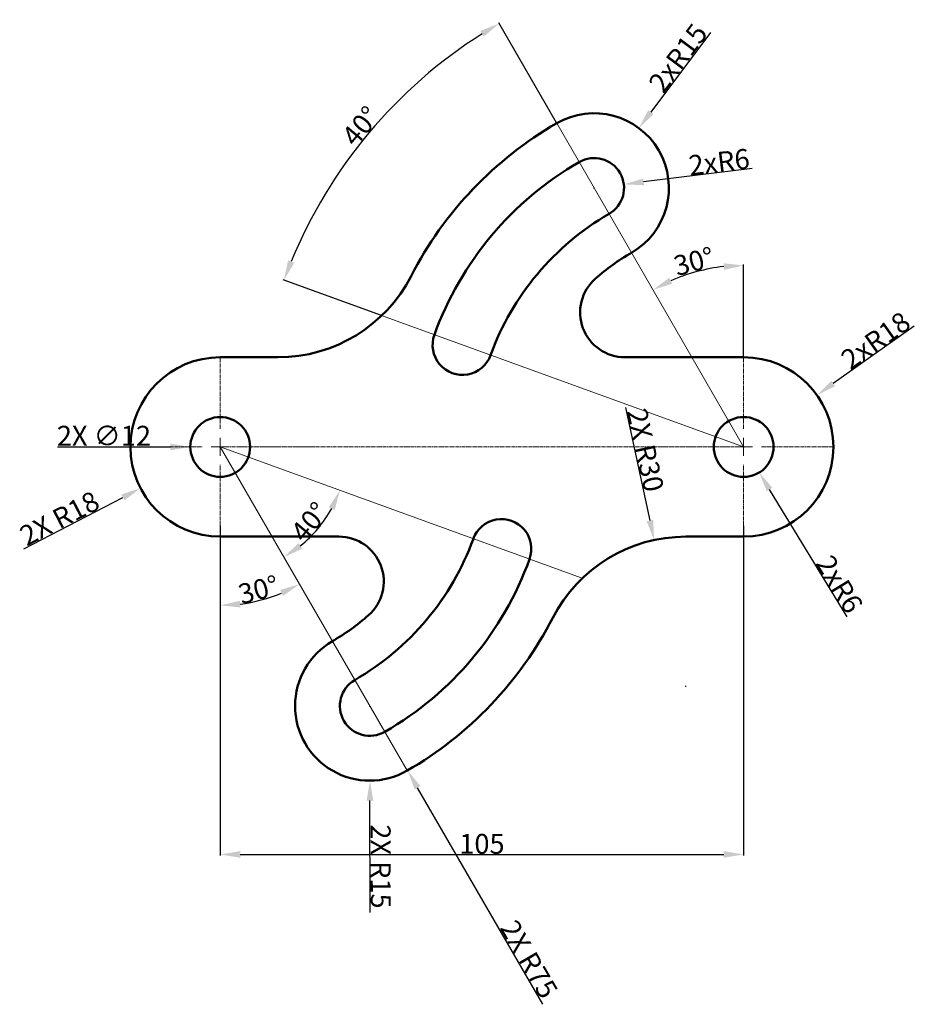
# Model space of a CAD drawing. Units: millimetres. Extents: x 75 to 254, y -22 to 175.
import ezdxf

# ---------------------------------------------------------------- set-up
doc = ezdxf.new("R2010")
doc.units = ezdxf.units.MM
doc.header["$MEASUREMENT"] = 0
doc.linetypes.add('CENTER2', pattern=[1.125, 0.75, -0.125, 0.125, -0.125])
for name, color, linetype, lineweight in [('M-CNTR', 8, 'CENTER2', 18), ('M-CONS', 8, 'Continuous', 13), ('M-DIMS', 2, 'Continuous', 25), ('M-OUTL', 7, 'Continuous', 50)]:
    doc.layers.add(name, color=color, linetype=linetype, lineweight=lineweight)
doc.styles.get("Standard").update_dxf_attribs({"font": 'arial.ttf'})
doc.dimstyles.get("Standard").update_dxf_attribs({"dimtxt": 4, "dimasz": 4, "dimexe": 0.18, "dimexo": 0.0625, "dimgap": 0.09, "dimtad": 1, "dimdec": 0, "dimzin": 0, "dimdsep": 46, "dimtxsty": 'Standard', "dimcen": 0.09, "dimclre": 251, "dimadec": 0, "dimazin": 0, "dimtfac": 1, "dimtdec": 0, "dimtofl": 0, "dimtmove": 0, "dimatfit": 3, "dimfxl": 1, "dimtolj": 1, "dimtzin": 0, "dimarcsym": 0})

# ---------------------------------------------------------------- blocks, each defined once
blk = doc.blocks.new('*U1')
at = {"layer": 'M-CNTR', "color": 0, "transparency": 16777216}
for p, q in [((0, 3.6), (0, 18.12)), ((-18.12, 0), (-3.6, 0)), ((3.6, 0), (18.12, 0)), ((0, -18.12), (0, -3.6))]:
    blk.add_line(p, q, dxfattribs=at)
at = {"layer": 'M-CNTR', "color": 0, "linetype": 'Continuous', "transparency": 16777216}
for p, q in [((-1.8, 0), (1.8, 0)), ((0, -1.8), (0, 1.8))]:
    blk.add_line(p, q, dxfattribs=at)
blk = doc.blocks.new('*U2')
at = {"layer": 'M-CNTR', "color": 0, "transparency": 16777216}
for p, q in [((0, 3.6), (0, 18.12)), ((-18.12, 0), (-3.6, 0)), ((3.6, 0), (18.12, 0)), ((0, -18.12), (0, -3.6))]:
    blk.add_line(p, q, dxfattribs=at)
at = {"layer": 'M-CNTR', "color": 0, "linetype": 'Continuous', "transparency": 16777216}
for p, q in [((-1.8, 0), (1.8, 0)), ((0, -1.8), (0, 1.8))]:
    blk.add_line(p, q, dxfattribs=at)
blk = doc.blocks.new('*D3')
at = {"layer": 'Defpoints', "color": 0, "transparency": 16777216}
for p in [(152.62, 160.91), (182.47, 154.53), (147.35, 115.92), (219.97, 89.58), (219.97, 89.58)]:
    blk.add_point(p, dxfattribs=at)
at = {"layer": 'M-DIMS', "color": 0, "lineweight": -2, "transparency": 16777216}
for p, q in [((182.44, 154.58), (170.83, 174.69)), ((147.29, 115.94), (127.58, 123.09))]:
    blk.add_line(p, q, dxfattribs=at)
blk.add_arc((219.97, 89.58), 98.1, 122.3363, 157.7248, dxfattribs=at)
at = {"layer": 'M-DIMS', "color": 0, "transparency": 16777216}
for points in [[(167.15, 173.04), (167.84, 171.9), (170.92, 174.54)], [(129.81, 126.52), (128.57, 127), (127.75, 123.03)]]:
    blk.add_solid(points, dxfattribs=at)
at = {"layer": 'M-DIMS', "color": 0, "transparency": 16777216, "insert": (143.15, 153.97), "char_height": 4, "attachment_point": 5, "rotation": 50.0305}
blk.add_mtext('\\A1;40°', dxfattribs=at)
blk = doc.blocks.new('*D4')
at = {"layer": 'Defpoints', "color": 0, "transparency": 16777216}
for p in [(114.97, 89.58), (114.97, 85.98), (114.97, 71.46), (120.49, 58.27), (152.47, 24.63)]:
    blk.add_point(p, dxfattribs=at)
at = {"layer": 'M-DIMS', "color": 0, "lineweight": -2, "transparency": 16777216}
blk.add_line((114.97, 71.39), (114.97, 57.61), dxfattribs=at)
blk.add_arc((114.97, 89.58), 31.79, 277.2151, 292.7849, dxfattribs=at)
at = {"layer": 'M-DIMS', "color": 0, "transparency": 16777216}
for points in [[(126.99, 60.87), (127.58, 59.68), (130.86, 62.05)], [(119.01, 57.38), (118.92, 58.71), (114.97, 57.79)]]:
    blk.add_solid(points, dxfattribs=at)
at = {"layer": 'M-DIMS', "color": 0, "transparency": 16777216, "insert": (122.65, 60.94), "char_height": 4, "attachment_point": 5, "rotation": 15}
blk.add_mtext('\\A1;30°', dxfattribs=at)
blk = doc.blocks.new('*D5')
at = {"layer": 'Defpoints', "color": 0, "transparency": 16777216}
for p in [(114.97, 89.58), (114.97, 89.58), (132.5, 71.01), (187.6, 63.23), (152.47, 24.63)]:
    blk.add_point(p, dxfattribs=at)
at = {"layer": 'M-DIMS', "color": 0, "lineweight": -2, "transparency": 16777216}
blk.add_arc((114.97, 89.58), 25.54, 308.9834, 331.0777, dxfattribs=at)
at = {"layer": 'M-DIMS', "color": 0, "transparency": 16777216}
for points in [[(136.72, 77.5), (137.93, 76.95), (138.98, 80.87)], [(131.42, 69.18), (130.66, 70.28), (127.74, 67.46)]]:
    blk.add_solid(points, dxfattribs=at)
at = {"layer": 'M-DIMS', "color": 0, "transparency": 16777216, "insert": (132.91, 74.54), "char_height": 4, "attachment_point": 5, "rotation": 50.0305}
blk.add_mtext('\\A1;40°', dxfattribs=at)
blk = doc.blocks.new('*D6')
at = {"layer": 'Defpoints', "color": 0, "transparency": 16777216}
for p in [(114.97, 73.82), (219.97, 73.82), (219.97, 7.81)]:
    blk.add_point(p, dxfattribs=at)
at = {"layer": 'M-DIMS', "color": 0, "lineweight": -2, "transparency": 16777216}
for p, q in [((114.97, 73.75), (114.97, 7.63)), ((219.97, 73.75), (219.97, 7.63)), ((118.97, 7.81), (215.97, 7.81))]:
    blk.add_line(p, q, dxfattribs=at)
at = {"layer": 'M-DIMS', "color": 0, "transparency": 16777216}
for points in [[(118.97, 8.48), (118.97, 7.15), (114.97, 7.81)], [(215.97, 8.48), (215.97, 7.15), (219.97, 7.81)]]:
    blk.add_solid(points, dxfattribs=at)
at = {"layer": 'M-DIMS', "color": 0, "transparency": 16777216, "insert": (167.47, 9.94), "char_height": 4, "attachment_point": 5}
blk.add_mtext('\\A1;105', dxfattribs=at)
blk = doc.blocks.new('*D7')
at = {"layer": 'Defpoints', "color": 0, "transparency": 16777216}
for p in [(234.66, 99.98), (219.97, 89.58)]:
    blk.add_point(p, dxfattribs=at)
at = {"layer": 'M-DIMS', "color": 0, "lineweight": -2, "transparency": 16777216}
for p, q in [((254.18, 113.81), (237.93, 102.29)), ((219.88, 89.58), (220.06, 89.58)), ((219.97, 89.49), (219.97, 89.67))]:
    blk.add_line(p, q, dxfattribs=at)
at = {"layer": 'M-DIMS', "color": 0, "transparency": 16777216}
blk.add_solid([(237.54, 102.84), (238.31, 101.75), (234.66, 99.98)], dxfattribs=at)
at = {"layer": 'M-DIMS', "color": 0, "transparency": 16777216, "insert": (246.45, 110.95), "char_height": 4, "attachment_point": 5, "rotation": 35.3084}
blk.add_mtext('\\A1;2xR18', dxfattribs=at)
blk = doc.blocks.new('*D8')
at = {"layer": 'Defpoints', "color": 0, "transparency": 16777216}
for p in [(219.97, 89.58), (223.09, 84.45)]:
    blk.add_point(p, dxfattribs=at)
at = {"layer": 'M-DIMS', "color": 0, "lineweight": -2, "transparency": 16777216}
for p, q in [((219.88, 89.58), (220.06, 89.58)), ((219.97, 89.49), (219.97, 89.67)), ((240.72, 55.46), (225.17, 81.03))]:
    blk.add_line(p, q, dxfattribs=at)
at = {"layer": 'M-DIMS', "color": 0, "transparency": 16777216}
blk.add_solid([(225.74, 81.38), (224.6, 80.69), (223.09, 84.45)], dxfattribs=at)
at = {"layer": 'M-DIMS', "color": 0, "transparency": 16777216, "insert": (239.21, 62.04), "char_height": 4, "attachment_point": 5, "rotation": 301.3002}
blk.add_mtext('\\A1;2xR6', dxfattribs=at)
blk = doc.blocks.new('*D9')
at = {"layer": 'Defpoints', "color": 0, "transparency": 16777216}
for p in [(182.47, 154.53), (213.65, 125.43), (219.97, 107.7), (219.97, 93.18), (219.97, 89.58)]:
    blk.add_point(p, dxfattribs=at)
at = {"layer": 'M-DIMS', "color": 0, "lineweight": -2, "transparency": 16777216}
blk.add_line((219.97, 107.76), (219.97, 126.17), dxfattribs=at)
blk.add_arc((219.97, 89.58), 36.41, 96.2977, 113.7023, dxfattribs=at)
at = {"layer": 'M-DIMS', "color": 0, "transparency": 16777216}
for points in [[(215.94, 126.43), (216.01, 125.1), (219.97, 125.99)], [(205.64, 122.32), (205.03, 123.51), (201.77, 121.11)]]:
    blk.add_solid(points, dxfattribs=at)
at = {"layer": 'M-DIMS', "color": 0, "transparency": 16777216, "insert": (210, 126.81), "char_height": 4, "attachment_point": 5, "rotation": 15}
blk.add_mtext('\\A1;30°', dxfattribs=at)
blk = doc.blocks.new('*D10')
at = {"layer": 'Defpoints', "color": 0, "transparency": 16777216}
for p in [(198.96, 153.55), (189.97, 141.54)]:
    blk.add_point(p, dxfattribs=at)
at = {"layer": 'M-DIMS', "color": 0, "lineweight": -2, "transparency": 16777216}
for p, q in [((213.3, 172.73), (201.35, 156.75)), ((189.88, 141.54), (190.06, 141.54)), ((189.97, 141.45), (189.97, 141.63))]:
    blk.add_line(p, q, dxfattribs=at)
at = {"layer": 'M-DIMS', "color": 0, "transparency": 16777216}
blk.add_solid([(200.82, 157.15), (201.88, 156.36), (198.96, 153.55)], dxfattribs=at)
at = {"layer": 'M-DIMS', "color": 0, "transparency": 16777216, "insert": (206.81, 167.62), "char_height": 4, "attachment_point": 5, "rotation": 53.2096}
blk.add_mtext('\\A1;2xR15', dxfattribs=at)
blk = doc.blocks.new('*D11')
at = {"layer": 'Defpoints', "color": 0, "transparency": 16777216}
for p in [(195.93, 142.27), (189.97, 141.54)]:
    blk.add_point(p, dxfattribs=at)
at = {"layer": 'M-DIMS', "color": 0, "lineweight": -2, "transparency": 16777216}
for p, q in [((221.66, 145.42), (199.9, 142.76)), ((189.88, 141.54), (190.06, 141.54)), ((189.97, 141.45), (189.97, 141.63))]:
    blk.add_line(p, q, dxfattribs=at)
at = {"layer": 'M-DIMS', "color": 0, "transparency": 16777216}
blk.add_solid([(199.82, 143.42), (199.98, 142.09), (195.93, 142.27)], dxfattribs=at)
at = {"layer": 'M-DIMS', "color": 0, "transparency": 16777216, "insert": (215.05, 146.76), "char_height": 4, "attachment_point": 5, "rotation": 6.9895}
blk.add_mtext('\\A1;2xR6', dxfattribs=at)
blk = doc.blocks.new('SLOT-ARC-R60-W12')
for centre, radius, start, end in [((32.4, 37.5), 6, 300, 120), ((62.4, -14.46), 66, 120, 160.0611), ((62.4, -14.46), 54, 120, 160.0611), ((6, 6), 6, 160.0611, 340.0611)]:
    blk.add_arc(centre, radius, start, end)
blk = doc.blocks.new('*D13')
at = {"layer": 'Defpoints', "color": 0, "transparency": 16777216}
for p in [(114.97, 89.58), (152.55, 24.67)]:
    blk.add_point(p, dxfattribs=at)
at = {"layer": 'M-DIMS', "color": 251, "lineweight": -2, "transparency": 16777216}
for p, q in [((114.88, 89.58), (115.06, 89.58)), ((114.97, 89.49), (114.97, 89.67))]:
    blk.add_line(p, q, dxfattribs=at)
at = {"layer": 'M-DIMS', "color": 0, "lineweight": -2, "transparency": 16777216}
blk.add_line((179.71, -22.25), (154.55, 21.21), dxfattribs=at)
at = {"layer": 'M-DIMS', "color": 0, "transparency": 16777216}
blk.add_solid([(155.13, 21.54), (153.97, 20.87), (152.55, 24.67)], dxfattribs=at)
at = {"layer": 'M-DIMS', "color": 0, "transparency": 16777216, "insert": (176.93, -13.21), "char_height": 4, "attachment_point": 5, "rotation": 300.0647}
blk.add_mtext('\\A1;2X R75', dxfattribs=at)
blk = doc.blocks.new('*D14')
at = {"layer": 'Defpoints', "color": 0, "transparency": 16777216}
for p in [(202.01, 70.9), (208.36, 41.58)]:
    blk.add_point(p, dxfattribs=at)
at = {"layer": 'M-DIMS', "color": 0, "lineweight": -2, "transparency": 16777216}
blk.add_line((196.26, 97.48), (201.16, 74.81), dxfattribs=at)
at = {"layer": 'M-DIMS', "color": 251, "lineweight": -2, "transparency": 16777216}
for p, q in [((208.27, 41.58), (208.45, 41.58)), ((208.36, 41.49), (208.36, 41.67))]:
    blk.add_line(p, q, dxfattribs=at)
at = {"layer": 'M-DIMS', "color": 0, "transparency": 16777216}
blk.add_solid([(201.82, 74.95), (200.51, 74.67), (202.01, 70.9)], dxfattribs=at)
at = {"layer": 'M-DIMS', "color": 0, "transparency": 16777216, "insert": (200.29, 88.94), "char_height": 4, "attachment_point": 5, "rotation": 282.2146}
blk.add_mtext('\\A1;2X R30', dxfattribs=at)
blk = doc.blocks.new('*D15')
at = {"layer": 'Defpoints', "color": 0, "transparency": 16777216}
for p in [(108.97, 89.58), (120.97, 89.58)]:
    blk.add_point(p, dxfattribs=at)
at = {"layer": 'M-DIMS', "color": 0, "lineweight": -2, "transparency": 16777216}
blk.add_line((82.3, 89.58), (104.97, 89.58), dxfattribs=at)
at = {"layer": 'M-DIMS', "color": 251, "lineweight": -2, "transparency": 16777216}
for p, q in [((114.88, 89.58), (115.06, 89.58)), ((114.97, 89.49), (114.97, 89.67))]:
    blk.add_line(p, q, dxfattribs=at)
at = {"layer": 'M-DIMS', "color": 0, "transparency": 16777216}
blk.add_solid([(104.97, 90.24), (104.97, 88.91), (108.97, 89.58)], dxfattribs=at)
at = {"layer": 'M-DIMS', "color": 0, "transparency": 16777216, "insert": (91.64, 91.82), "char_height": 4, "attachment_point": 5, "rotation": 0.003}
blk.add_mtext('\\A1;2X ∅12', dxfattribs=at)
blk = doc.blocks.new('*D16')
at = {"layer": 'Defpoints', "color": 0, "transparency": 16777216}
for p in [(114.97, 89.58), (98.99, 81.3)]:
    blk.add_point(p, dxfattribs=at)
at = {"layer": 'M-DIMS', "color": 251, "lineweight": -2, "transparency": 16777216}
for p, q in [((114.88, 89.58), (115.06, 89.58)), ((114.97, 89.49), (114.97, 89.67))]:
    blk.add_line(p, q, dxfattribs=at)
at = {"layer": 'M-DIMS', "color": 0, "lineweight": -2, "transparency": 16777216}
blk.add_line((75.54, 69.14), (95.44, 79.45), dxfattribs=at)
at = {"layer": 'M-DIMS', "color": 0, "transparency": 16777216}
blk.add_solid([(95.13, 80.05), (95.75, 78.86), (98.99, 81.3)], dxfattribs=at)
at = {"layer": 'M-DIMS', "color": 0, "transparency": 16777216, "insert": (82.73, 75.27), "char_height": 4, "attachment_point": 5, "rotation": 27.3947}
blk.add_mtext('\\A1;2X R18', dxfattribs=at)
blk = doc.blocks.new('*D17')
at = {"layer": 'Defpoints', "color": 0, "transparency": 16777216}
for p in [(144.97, 37.62), (145, 22.62)]:
    blk.add_point(p, dxfattribs=at)
at = {"layer": 'M-DIMS', "color": 251, "lineweight": -2, "transparency": 16777216}
for p, q in [((144.88, 37.62), (145.06, 37.62)), ((144.97, 37.53), (144.97, 37.71))]:
    blk.add_line(p, q, dxfattribs=at)
at = {"layer": 'M-DIMS', "color": 0, "lineweight": -2, "transparency": 16777216}
blk.add_line((145.05, -3.82), (145.01, 18.62), dxfattribs=at)
at = {"layer": 'M-DIMS', "color": 0, "transparency": 16777216}
blk.add_solid([(145.67, 18.62), (144.34, 18.61), (145, 22.62)], dxfattribs=at)
at = {"layer": 'M-DIMS', "color": 0, "transparency": 16777216, "insert": (147.16, 5.4), "char_height": 4, "attachment_point": 5, "rotation": 270.1063}
blk.add_mtext('\\A1;2X R15', dxfattribs=at)

msp = doc.modelspace()

# ---------------------------------------------------------------- linework, layer by layer
at = {"layer": 'M-CNTR'}
msp.add_line((114.97, 89.58), (219.97, 89.58), dxfattribs=at)
at = {"layer": 'M-CONS'}
for p, q in [((219.97, 89.58), (182.47, 154.53)), ((219.97, 89.58), (147.35, 115.92)), ((114.97, 89.58), (152.47, 24.63)), ((114.97, 89.58), (187.6, 63.23))]:
    msp.add_line(p, q, dxfattribs=at)
at = {"layer": 'M-OUTL'}
for p, q in [((114.97, 107.58), (126.59, 107.58)), ((219.97, 107.58), (196.16, 107.58)), ((114.97, 71.58), (138.78, 71.58)), ((219.97, 71.58), (208.36, 71.58))]:
    msp.add_line(p, q, dxfattribs=at)
for centre in [(114.97, 89.58), (219.97, 89.58)]:
    msp.add_circle(centre, 6, dxfattribs=at)
for centre, radius, start, end in [((189.97, 141.54), 15, 300, 120), ((219.97, 89.58), 75, 120, 152.7971), ((219.97, 89.58), 45, 120, 131.4096), ((126.59, 137.58), 30, 270, 332.7971), ((196.16, 116.58), 9, 131.4096, 270), ((114.97, 89.58), 18, 90, 270), ((219.97, 89.58), 18, 270, 90), ((138.78, 62.58), 9, 311.4096, 90), ((208.36, 41.58), 30, 90, 152.7971), ((114.97, 89.58), 45, 300, 311.4096), ((114.97, 89.58), 75, 300, 332.7971), ((144.97, 37.62), 15, 120, 300)]:
    msp.add_arc(centre, radius, start, end, dxfattribs=at)

# ---------------------------------------------------------------- block references
at = {"layer": 'M-CNTR'}
for name, p in [('*U1', (114.97, 89.58)), ('*U2', (219.97, 89.58))]:
    msp.add_blockref(name, p, dxfattribs=at)
at = {"layer": 'M-OUTL'}
msp.add_blockref('SLOT-ARC-R60-W12', (157.57, 104.04), dxfattribs=at)
at = {"layer": 'M-OUTL', "rotation": 180}
msp.add_blockref('SLOT-ARC-R60-W12', (177.38, 75.12), dxfattribs=at)

# ---------------------------------------------------------------- dimensions: what is measured, and where the dimension line sits
at = {"layer": 'M-DIMS'}
for base, line1, line2, picture, middle in [((152.62, 160.91), ((219.97, 89.58), (182.47, 154.53)), ((219.97, 89.58), (147.35, 115.92)), '*D3', (143.15, 153.97)), ((213.65, 125.43), ((219.97, 93.18), (219.97, 107.7)), ((219.97, 89.58), (182.47, 154.53)), '*D9', (210, 126.81)), ((120.49, 58.27), ((114.97, 89.58), (152.47, 24.63)), ((114.97, 71.46), (114.97, 85.98)), '*D4', (122.65, 60.94)), ((132.5, 71.01), ((114.97, 89.58), (187.6, 63.23)), ((114.97, 89.58), (152.47, 24.63)), '*D5', (132.91, 74.54))]:
    dim = msp.add_angular_dim_2l(base=base, line1=line1, line2=line2, dimstyle='Standard', override={"dimclrd": 0, "dimclre": 0, "dimclrt": 0}, dxfattribs=at)
    dim.commit()
    dim.dimension.update_dxf_attribs({"geometry": picture, "text_midpoint": middle})
for center, mpoint, text, override, picture, middle in [((189.97, 141.54), (198.96, 153.55), '2x<>', {"dimclrd": 0, "dimclre": 0, "dimclrt": 0}, '*D10', (206.81, 167.62)), ((219.97, 89.58), (234.66, 99.98), '2x<>', {"dimclrd": 0, "dimclre": 0, "dimclrt": 0}, '*D7', (246.45, 110.95)), ((114.97, 89.58), (98.99, 81.3), '2X <>', {"dimdec": 0, "dimlfac": 1, "dimrnd": 0, "dimzin": 0, "dimdsep": 46, "dimlunit": 2}, '*D16', (82.73, 75.27)), ((144.97, 37.62), (145, 22.62), '2X <>', {"dimdec": 0, "dimlfac": 1, "dimrnd": 0, "dimzin": 0, "dimdsep": 46, "dimlunit": 2}, '*D17', (147.16, 5.4))]:
    dim = msp.add_radius_dim(center=center, mpoint=mpoint, text=text, dimstyle='Standard', override=override, dxfattribs=at)
    dim.commit()
    dim.dimension.update_dxf_attribs({"geometry": picture, "text_midpoint": middle})
for center, mpoint, text, override, picture, middle in [((189.97, 141.54), (195.93, 142.27), '2x<>', {"dimclrd": 0, "dimclre": 0, "dimclrt": 0}, '*D11', (215.31, 144.64)), ((208.36, 41.58), (202.01, 70.9), '2X <>', {"dimdec": 0, "dimlfac": 1, "dimrnd": 0, "dimzin": 0, "dimdsep": 46, "dimlunit": 2}, '*D14', (198.2, 88.49)), ((114.97, 89.58), (152.55, 24.67), '2X <>', {"dimdec": 0, "dimlfac": 1, "dimrnd": 0, "dimzin": 0, "dimdsep": 46, "dimlunit": 2}, '*D13', (175.09, -14.28)), ((219.97, 89.58), (223.09, 84.45), '2x<>', {"dimclrd": 0, "dimclre": 0, "dimclrt": 0}, '*D8', (237.39, 60.93))]:
    dim = msp.add_radius_dim(center=center, mpoint=mpoint, text=text, dimstyle='Standard', override=override, dxfattribs=at)
    dim.commit()
    dim.dimension.update_dxf_attribs({"geometry": picture, "text_midpoint": middle, "dimtype": 164})
dim = msp.add_diameter_dim_2p(p1=(120.97, 89.58), p2=(108.97, 89.58), text='2X <>', dimstyle='Standard', override={"dimdec": 0, "dimlfac": 1, "dimrnd": 0, "dimzin": 0, "dimdsep": 46, "dimlunit": 2}, dxfattribs=at)
dim.commit()
dim.dimension.update_dxf_attribs({"geometry": '*D15', "text_midpoint": (91.64, 89.58), "dimtype": 163})
dim = msp.add_linear_dim(base=(219.97, 7.81), p1=(114.97, 73.82), p2=(219.97, 73.82), dimstyle='Standard', override={"dimclrd": 0, "dimclre": 0, "dimclrt": 0}, dxfattribs=at)
dim.commit()
dim.dimension.update_dxf_attribs({"geometry": '*D6', "text_midpoint": (167.47, 9.94)})

doc.saveas('drawing.dxf')
